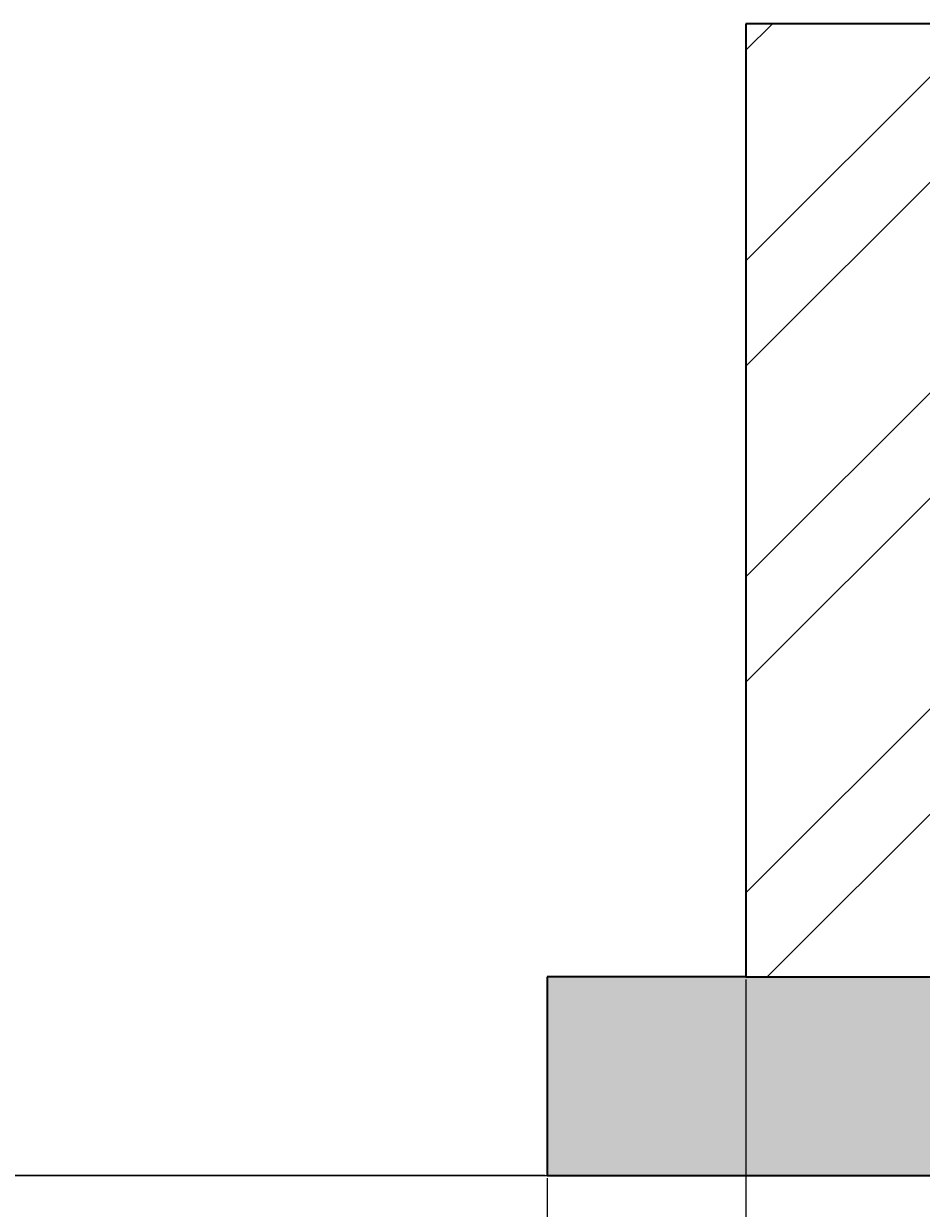
# Model space of a CAD drawing. Units: inches. Extents: x -301 to 715, y -607 to 364.
# Tile 28 of 141: x 101 to 124, y -541 to -511. Entities that reach past the tile are written whole.
import ezdxf

# ---------------------------------------------------------------- set-up
doc = ezdxf.new("R2010")
doc.units = ezdxf.units.IN
doc.header["$MEASUREMENT"] = 0
for name, color, linetype, lineweight in [('A-ANNO-DIMS', 2, 'Continuous', 18), ('A-SECT-PATT', 8, 'Continuous', 13), ('S-FNDN', 2, 'Continuous', 35)]:
    doc.layers.add(name, color=color, linetype=linetype, lineweight=lineweight)
doc.styles.get("Standard").update_dxf_attribs({"font": 'arial.ttf'})
doc.dimstyles.get("Standard").update_dxf_attribs({"dimtxt": 0.18, "dimasz": 0.18, "dimexe": 0.18, "dimexo": 0.0625, "dimgap": 0.09, "dimtad": 0, "dimtih": 1, "dimtoh": 1, "dimdec": 1, "dimzin": 0, "dimdsep": 46, "dimlunit": 4, "dimtxsty": 'Standard', "dimcen": 0.09, "dimclrd": 3, "dimclre": 4, "dimclrt": 6, "dimadec": 0, "dimazin": 0, "dimtfac": 1, "dimtdec": 1, "dimtofl": 0, "dimtmove": 0, "dimatfit": 3, "dimfxl": 1, "dimtfill": 2, "dimtfillclr": 51, "dimtolj": 1, "dimtzin": 0, "dimarcsym": 0})

# ---------------------------------------------------------------- blocks, each defined once
blk = doc.blocks.new('*D176')
at = {"layer": 'A-ANNO-DIMS', "color": 4, "lineweight": -2, "transparency": 16777216}
for p, q in [((148.28, -324.477), (215.605, -324.477)), ((-15.22, -540.477), (215.605, -540.477))]:
    blk.add_line(p, q, dxfattribs=at)
at = {"layer": 'A-ANNO-DIMS', "color": 3, "lineweight": -2, "transparency": 16777216}
for p, q in [((215.425, -324.657), (215.425, -432.296)), ((215.425, -540.297), (215.425, -432.659))]:
    blk.add_line(p, q, dxfattribs=at)
at = {"layer": 'A-ANNO-DIMS', "color": 3, "transparency": 16777216}
for points in [[(215.395, -324.657), (215.455, -324.657), (215.425, -324.477)], [(215.395, -540.297), (215.455, -540.297), (215.425, -540.477)]]:
    blk.add_solid(points, dxfattribs=at)
at = {"layer": 'Defpoints', "color": 0, "transparency": 16777216}
for p in [(148.218, -324.477), (-15.282, -540.477), (215.425, -540.477)]:
    blk.add_point(p, dxfattribs=at)
at = {"layer": 'A-ANNO-DIMS', "color": 6, "transparency": 16777216, "insert": (215.425, -432.477), "char_height": 0.18, "attachment_point": 5, "bg_fill": 1, "box_fill_scale": 1.25, "bg_fill_color": 51, "bg_fill_transparency": 0}
blk.add_mtext('\\A1;18\'-0"', dxfattribs=at)
blk = doc.blocks.new('*D182')
at = {"layer": 'A-ANNO-DIMS', "color": 4, "lineweight": -2, "transparency": 16777216}
for p, q in [((114.255, -540.54), (114.255, -573.809)), ((163.255, -540.54), (163.255, -573.809))]:
    blk.add_line(p, q, dxfattribs=at)
at = {"layer": 'A-ANNO-DIMS', "color": 3, "lineweight": -2, "transparency": 16777216}
for p, q in [((114.435, -573.629), (138.422, -573.629)), ((163.075, -573.629), (139.088, -573.629))]:
    blk.add_line(p, q, dxfattribs=at)
at = {"layer": 'A-ANNO-DIMS', "color": 3, "transparency": 16777216}
for points in [[(114.435, -573.599), (114.435, -573.659), (114.255, -573.629)], [(163.075, -573.599), (163.075, -573.659), (163.255, -573.629)]]:
    blk.add_solid(points, dxfattribs=at)
at = {"layer": 'Defpoints', "color": 0, "transparency": 16777216}
for p in [(114.255, -540.477), (163.255, -540.477), (163.255, -573.629)]:
    blk.add_point(p, dxfattribs=at)
at = {"layer": 'A-ANNO-DIMS', "color": 6, "transparency": 16777216, "insert": (138.755, -573.629), "char_height": 0.18, "attachment_point": 5, "bg_fill": 1, "box_fill_scale": 1.25, "bg_fill_color": 51, "bg_fill_transparency": 0}
blk.add_mtext('\\A1;4\'-1"', dxfattribs=at)
blk = doc.blocks.new('*D183')
at = {"layer": 'A-ANNO-DIMS', "color": 4, "lineweight": -2, "transparency": 16777216}
for p, q in [((119.255, -535.54), (119.255, -573.809)), ((158.255, -535.54), (158.255, -573.809))]:
    blk.add_line(p, q, dxfattribs=at)
at = {"layer": 'A-ANNO-DIMS', "color": 3, "lineweight": -2, "transparency": 16777216}
for p, q in [((119.435, -573.629), (138.426, -573.629)), ((158.075, -573.629), (139.084, -573.629))]:
    blk.add_line(p, q, dxfattribs=at)
at = {"layer": 'A-ANNO-DIMS', "color": 3, "transparency": 16777216}
for points in [[(119.435, -573.599), (119.435, -573.659), (119.255, -573.629)], [(158.075, -573.599), (158.075, -573.659), (158.255, -573.629)]]:
    blk.add_solid(points, dxfattribs=at)
at = {"layer": 'Defpoints', "color": 0, "transparency": 16777216}
for p in [(119.255, -535.477), (158.255, -535.477), (158.255, -573.629)]:
    blk.add_point(p, dxfattribs=at)
at = {"layer": 'A-ANNO-DIMS', "color": 6, "transparency": 16777216, "insert": (138.755, -573.629), "char_height": 0.18, "attachment_point": 5, "bg_fill": 1, "box_fill_scale": 1.25, "bg_fill_color": 51, "bg_fill_transparency": 0}
blk.add_mtext('\\A1;3\'-3"', dxfattribs=at)
blk = doc.blocks.new('*D191')
at = {"layer": 'A-ANNO-DIMS', "color": 4, "lineweight": -2, "transparency": 16777216}
for p, q in [((129.193, -481.477), (-266.112, -481.477)), ((114.193, -540.477), (-266.112, -540.477))]:
    blk.add_line(p, q, dxfattribs=at)
at = {"layer": 'A-ANNO-DIMS', "color": 3, "lineweight": -2, "transparency": 16777216}
for p, q in [((-265.932, -481.657), (-265.932, -510.797)), ((-265.932, -540.297), (-265.932, -511.158))]:
    blk.add_line(p, q, dxfattribs=at)
at = {"layer": 'A-ANNO-DIMS', "color": 3, "transparency": 16777216}
for points in [[(-265.962, -481.657), (-265.902, -481.657), (-265.932, -481.477)], [(-265.962, -540.297), (-265.902, -540.297), (-265.932, -540.477)]]:
    blk.add_solid(points, dxfattribs=at)
at = {"layer": 'Defpoints', "color": 0, "transparency": 16777216}
for p in [(129.255, -481.477), (-265.932, -540.477), (114.255, -540.477)]:
    blk.add_point(p, dxfattribs=at)
at = {"layer": 'A-ANNO-DIMS', "color": 6, "transparency": 16777216, "insert": (-265.932, -510.977), "char_height": 0.18, "attachment_point": 5, "bg_fill": 1, "box_fill_scale": 1.25, "bg_fill_color": 51, "bg_fill_transparency": 0}
blk.add_mtext('\\A1;4\'-11"', dxfattribs=at)

msp = doc.modelspace()

# ---------------------------------------------------------------- hatches: boundary and pattern name
at = {"layer": 'A-SECT-PATT'}
h = msp.add_hatch(dxfattribs=at)
h.set_pattern_fill('ANSI32', color=256, scale=15)
h.set_pattern_definition([(45, (10.321, 33.8764), (-3.977476, 3.977476), []), (45, (12.973, 33.8764), (-3.977476, 3.977476), [])])
h.paths.add_polyline_path([(-185.282, -324.477), (-199.282, -324.477), (-199.282, -329.477), (-194.282, -329.477), (-194.282, -353.477), (-185.282, -353.477)])
h.paths.add_polyline_path([(-185.282, -361.477), (-193.904, -361.477), (-193.982, -377.537), (-185.282, -377.537)])
h.paths.add_polyline_path([(143.218, -329.477), (148.218, -329.477), (148.218, -324.477), (134.255, -324.477), (134.255, -353.477), (143.218, -353.477)])
h.paths.add_polyline_path([(143.218, -361.477), (134.255, -361.477), (134.255, -377.477), (143.218, -377.477)])
h.paths.add_polyline_path([(-185.282, -439.477), (-194.282, -439.477), (-194.282, -463.477), (-185.282, -463.477)])
h.paths.add_polyline_path([(-185.282, -471.477), (-194.282, -471.477), (-194.282, -481.477), (-185.282, -481.477)])
h.paths.add_polyline_path([(-185.282, -463.477), (-194.282, -463.477), (-194.282, -466.477), (-185.282, -466.477)])
h.paths.add_polyline_path([(-185.282, -466.477), (-194.282, -466.477), (-194.282, -471.477), (-185.282, -471.477)])
h.paths.add_polyline_path([(-180.282, -481.477), (-185.282, -481.477), (-194.282, -481.477), (-199.282, -481.477), (-199.282, -493.477), (-180.282, -493.477)])
h.paths.add_polyline_path([(-175.282, -493.477), (-180.282, -493.477), (-199.282, -493.477), (-204.282, -493.477), (-204.282, -511.477), (-175.282, -511.477)])
h.paths.add_polyline_path([(-170.282, -511.477), (-175.282, -511.477), (-204.282, -511.477), (-209.282, -511.477), (-209.282, -535.477), (-170.282, -535.477)])
h.paths.add_polyline_path([(-35.282, -463.477), (-41.282, -463.477), (-41.282, -466.477), (-35.282, -466.477)])
h.paths.add_polyline_path([(-35.282, -466.477), (-41.282, -466.477), (-41.282, -471.477), (-35.282, -471.477)])
h.paths.add_polyline_path([(-35.282, -471.477), (-41.282, -471.477), (-41.282, -481.477), (-35.282, -481.477)])
h.paths.add_polyline_path([(-30.282, -481.477), (-46.282, -481.477), (-46.282, -493.477), (-30.282, -493.477)])
h.paths.add_polyline_path([(-25.282, -493.477), (-30.282, -493.477), (-46.282, -493.477), (-51.282, -493.477), (-51.282, -511.477), (-25.282, -511.477)])
h.paths.add_polyline_path([(-20.282, -511.477), (-25.282, -511.477), (-51.282, -511.477), (-56.282, -511.477), (-56.282, -535.477), (-20.282, -535.477)])
h.paths.add_polyline_path([(143.218, -463.477), (134.255, -463.477), (134.255, -466.477), (143.218, -466.477)])
h.paths.add_polyline_path([(143.218, -466.477), (134.255, -466.477), (134.255, -471.477), (143.218, -471.477)])
h.paths.add_polyline_path([(143.218, -471.477), (134.255, -471.477), (134.255, -481.477), (143.218, -481.477)])
h.paths.add_polyline_path([(148.255, -481.477), (143.255, -481.477), (134.255, -481.477), (129.255, -481.477), (129.255, -493.477), (148.255, -493.477)])
h.paths.add_polyline_path([(153.255, -493.477), (148.255, -493.477), (129.255, -493.477), (124.255, -493.477), (124.255, -511.477), (153.255, -511.477)])
h.paths.add_polyline_path([(158.255, -511.477), (153.255, -511.477), (124.255, -511.477), (119.255, -511.477), (119.255, -535.477), (158.255, -535.477)])
h = msp.add_hatch(dxfattribs=at)
h.set_pattern_fill('AR-CONC', color=256, scale=0.5)
h.set_pattern_definition([(50, (10.3213, 33.8764), (3.586301, -0.31376), [0.375, -4.125]), (355, (10.3213, 33.8764), (-0.693757, 3.76096), [0.3, -3.3]), (100.45144, (10.62, 33.8502), (2.892544, 3.4472), [0.3187, -3.50571]), (46.1842, (10.3213, 34.8764), (5.336207, -0.827596), [0.5625, -6.1875]), (96.6356, (10.766, 34.8074), (4.67331, 4.870593), [0.47805, -5.25857]), (351.1842, (10.321, 34.8764), (4.67331, 4.870593), [0.45, -4.95]), (21, (10.8213, 34.6264), (2.984535, -2.013094), [0.375, -4.125]), (326, (10.8213, 34.6264), (1.216577, 3.62575), [0.3, -3.3]), (71.45144, (11.07, 34.4586), (4.201112, 1.612656), [0.3187, -3.50571]), (37.5, (10.3213, 33.8764), (0.0607993, 1.6644693), [0, -3.26, 0, -3.35, 0, -3.3125]), (7.5, (10.3213, 33.8764), (1.3153477, 1.9720586), [0, -1.91, 0, -3.185, 0, -1.2625]), (327.5, (9.2063, 33.8764), (2.6691122, -0.1127744), [0, -1.25, 0, -3.9, 0, -5.175]), (317.5, (8.7063, 33.8764), (2.915931, 0.500525), [0, -1.625, 0, -2.59, 0, -3.675])])
h.paths.add_polyline_path([(-56.282, -535.477), (-61.282, -535.477), (-61.282, -540.477), (-15.282, -540.477), (-15.282, -535.477), (-20.282, -535.477)])
h.paths.add_polyline_path([(119.255, -535.477), (114.255, -535.477), (114.255, -540.477), (163.255, -540.477), (163.255, -535.477), (158.255, -535.477)])
h.paths.add_polyline_path([(-206.282, -471.477), (-209.282, -471.477), (-209.282, -481.477), (-206.282, -481.477), (-194.282, -481.477), (-194.282, -471.477)])
h.paths.add_polyline_path([(-41.282, -481.477), (-41.282, -471.477), (-185.282, -471.477), (-185.282, -481.477), (-180.282, -481.477)])
h.paths.add_polyline_path([(134.255, -481.477), (134.255, -471.477), (-35.282, -471.477), (-35.282, -481.477), (-30.282, -481.477)])
h.paths.add_polyline_path([(155.218, -481.477), (158.218, -481.477), (158.218, -471.477), (153.218, -471.477), (143.218, -471.477), (143.218, -481.477), (148.255, -481.477)])
h.paths.add_polyline_path([(-193.88, -356.477), (-193.904, -361.477), (143.218, -361.477), (143.218, -356.477)])

# ---------------------------------------------------------------- linework, layer by layer
at = {"layer": 'S-FNDN'}
for p, q in [((124.255, -511.477), (119.255, -511.477)), ((119.255, -511.477), (119.255, -535.477)), ((119.255, -535.477), (114.255, -535.477)), ((114.255, -535.477), (114.255, -540.477)), ((119.255, -535.477), (158.255, -535.477)), ((114.255, -540.477), (163.255, -540.477))]:
    msp.add_line(p, q, dxfattribs=at)

# ---------------------------------------------------------------- dimensions: what is measured, and where the dimension line sits
at = {"layer": 'A-ANNO-DIMS'}
for base, p1, p2, picture, middle in [((215.425, -540.477), (148.218, -324.477), (-15.282, -540.477), '*D176', (215.425, -432.477)), ((-265.932, -540.477), (129.255, -481.477), (114.255, -540.477), '*D191', (-265.932, -510.977))]:
    dim = msp.add_linear_dim(base=base, p1=p1, p2=p2, angle=90, dimstyle='Standard', override={"dimdec": 1, "dimlfac": 1, "dimrnd": 0, "dimzin": 1, "dimdsep": 46, "dimlunit": 4, "dimfrac": 2}, dxfattribs=at)
    dim.commit()
    dim.dimension.update_dxf_attribs({"geometry": picture, "text_midpoint": middle})
for base, p1, p2, picture in [((158.255, -573.629), (119.255, -535.477), (158.255, -535.477), '*D183'), ((163.255, -573.629), (114.255, -540.477), (163.255, -540.477), '*D182')]:
    dim = msp.add_linear_dim(base=base, p1=p1, p2=p2, dimstyle='Standard', override={"dimdec": 1, "dimlfac": 1, "dimrnd": 0, "dimzin": 1, "dimdsep": 46, "dimlunit": 4, "dimfrac": 2}, dxfattribs=at)
    dim.commit()
    dim.dimension.update_dxf_attribs({"geometry": picture, "text_midpoint": (138.755, -573.629)})

doc.saveas('drawing.dxf')
